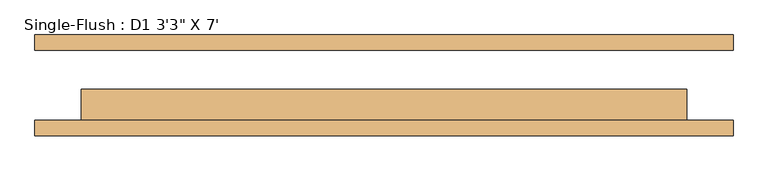
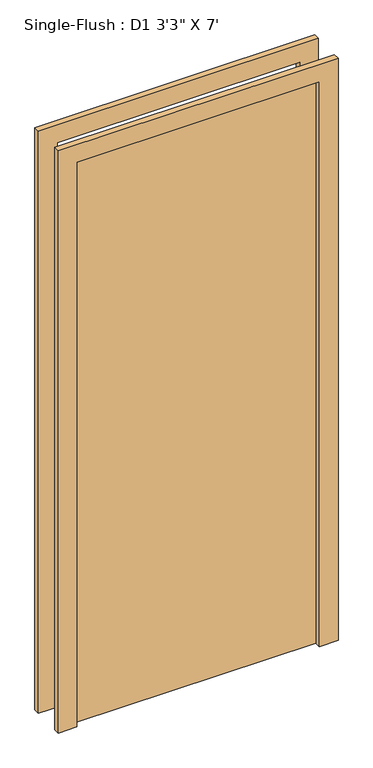
"""IFC4 building model written with IfcOpenShell, lengths in millimetres: door geometry."""

from ifc_helpers import new_model, si_unit, frame, origin, origin_with_axes, place, context, project, spatial, polyline, outline, extrude, source, transform, mapped, element, save


def door_3ddad2be(model_context):
    return source(origin(), model_context, "Body", "SweptSolid", [
        extrude(outline(polyline([(2514.6, -571.5), (0.0, -571.5), (0.0, -495.3), (2438.4, -495.3), (2438.4, 495.3), (0.0, 495.3), (0.0, 571.5), (2514.6, 571.5), (2514.6, -571.5)])), frame((0.0, -82.55, 0.0), z_axis=(0.0, 1.0, 0.0), x_axis=(0.0, 0.0, 1.0)), (0.0, 0.0, 1.0), 25.4),
        extrude(outline(polyline([(2514.6, 571.5), (2514.6, -571.5), (0.0, -571.5), (0.0, -495.3), (2438.4, -495.3), (2438.4, 495.3), (0.0, 495.3), (0.0, 571.5), (2514.6, 571.5)])), frame((0.0, 57.15, 0.0), z_axis=(0.0, 1.0, 0.0), x_axis=(0.0, 0.0, 1.0)), (0.0, 0.0, 1.0), 25.4),
        extrude(outline(polyline([(495.3, -6.35), (495.3, -57.15), (-495.3, -57.15), (-495.3, -6.35), (495.3, -6.35)])), origin_with_axes(), (0.0, 0.0, 1.0), 2438.4),
    ])


if __name__ == "__main__":
    model = new_model("IFC4")
    model_context = context("Model", 3, world=origin())
    ifc_project = project(units=[si_unit("LENGTHUNIT", "METRE", prefix="MILLI")], contexts=[model_context])
    site = spatial("IfcSite", under=ifc_project)
    building = spatial("IfcBuilding", under=site)
    placement = place(None, origin())
    door_shape = door_3ddad2be(model_context)
    element("IfcDoor", 1, ObjectType="Single-Flush : D1 3'3\" X 7'", at=placement, inside=building, context=model_context, shape_type="MappedRepresentation", body=[
        mapped(door_shape, transform((0.0, 0.0, 0.0), x_axis=(1.0, 0.0, 0.0), y_axis=(0.0, 1.0, 0.0), z_axis=(0.0, 0.0, 1.0))),
    ])
    save(model, "model.ifc")

# Revit data of these elements
# Type "Single-Flush : D1 3'3\" X 7'"
#   Type Mark = "9"
#   Construction Type Id = "MDOOR"
#   Assembly Code = "C1020"
#   Analytic Construction = "Metal"
#   Thickness = 0' - 2"
#   Heat Transfer Coefficient (U) = 0.651978 BTU/(h·ft²·°F)
#   Height = 8' - 0"
#   Trim Projection Ext = 0' - 1"
#   Trim Projection Int = 0' - 1"
#   Trim Width = 0' - 3"
#   Width = 3' - 3"
#   Define Thermal Properties by = 1
#   Door Material = Door - Panel
#   Frame Material = Door - Frame
#   Visual Light Transmittance = 0
#   Solar Heat Gain Coefficient = 0
#   Function = (empty or 0)
#   Wall Closure = (empty or 0)
# Element 1 (IfcDoor, "Single-Flush : D1 3'3\" X 7'")
#   Materials on its faces: "Door - Frame", "Door - Panel"
# Materials
#   "Door - Panel": class "Wood", colour RGB 210 159 95, transparency 0, Cost = 0
#   "Door - Frame": colour RGB 118 70 51, transparency 0, Cost = 0
